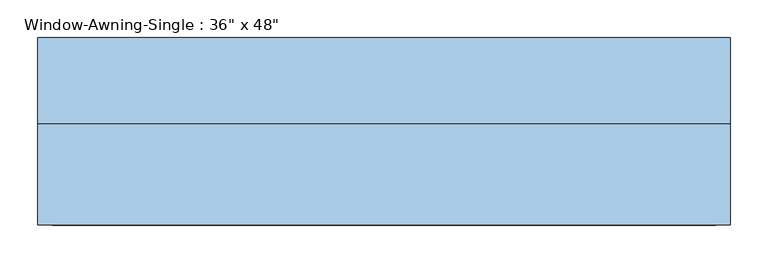
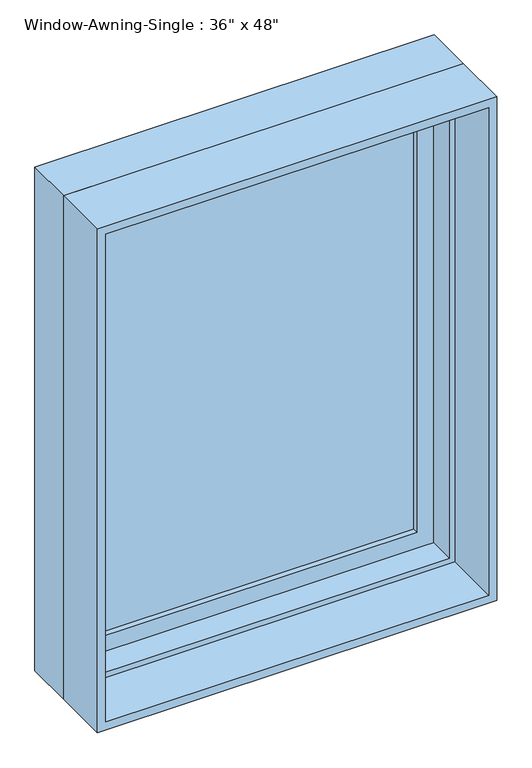
"""IFC4 building model written with IfcOpenShell, lengths in millimetres: window geometry."""

from ifc_helpers import new_model, si_unit, frame, origin, place, context, project, spatial, polyline, outline, extrude, faceted_brep, source, transform, mapped, element, save


def window_272f20d6(model_context):
    return source(origin(), model_context, "Body", "SolidModel", [
        extrude(outline(polyline([(2133.6, -457.2), (914.4, -457.2), (914.4, 457.2), (2133.6, 457.2), (2133.6, -457.2)]), holes=[polyline([(2114.55, -438.15), (2114.55, 438.15), (933.45, 438.15), (933.45, -438.15), (2114.55, -438.15)])]), frame((0.0, -114.3, 0.0), z_axis=(0.0, 1.0, 0.0), x_axis=(0.0, 0.0, 1.0)), (0.0, 0.0, 1.0), 133.35),
        extrude(outline(polyline([(927.1, -444.5), (927.1, 444.5), (2120.9, 444.5), (2120.9, -444.5), (927.1, -444.5)]), holes=[polyline([(2063.75, -387.35), (2063.75, 387.35), (984.25, 387.35), (984.25, -387.35), (2063.75, -387.35)])]), frame((0.0, 82.55, 0.0), z_axis=(0.0, 1.0, 0.0), x_axis=(0.0, 0.0, 1.0)), (0.0, 0.0, 1.0), 44.45),
        extrude(outline(polyline([(387.35, 114.3), (387.35, 107.95), (-387.35, 107.95), (-387.35, 114.3), (387.35, 114.3)])), frame((0.0, 0.0, 984.25), z_axis=(0.0, 0.0, 1.0), x_axis=(1.0, 0.0, 0.0)), (0.0, 0.0, 1.0), 1079.5),
        extrude(outline(polyline([(387.35, 101.6), (387.35, 95.25), (-387.35, 95.25), (-387.35, 101.6), (387.35, 101.6)])), frame((0.0, 0.0, 984.25), z_axis=(0.0, 0.0, 1.0), x_axis=(1.0, 0.0, 0.0)), (0.0, 0.0, 1.0), 1079.5),
        faceted_brep([(444.5, 82.55, 927.1), (444.5, 133.35, 927.1), (-444.5, 133.35, 927.1), (-444.5, 82.55, 927.1), (425.45, 19.05, 946.15), (425.45, 82.55, 946.15), (-425.45, 82.55, 946.15), (-425.45, 19.05, 946.15), (457.2, 133.35, 914.4), (457.2, 19.05, 914.4), (-457.2, 19.05, 914.4), (-457.2, 133.35, 914.4), (-444.5, 133.35, 2120.9), (-444.5, 82.55, 2120.9), (-425.45, 82.55, 2101.85), (-425.45, 19.05, 2101.85), (-457.2, 19.05, 2133.6), (-457.2, 133.35, 2133.6), (444.5, 133.35, 2120.9), (444.5, 82.55, 2120.9), (425.45, 82.55, 2101.85), (425.45, 19.05, 2101.85), (457.2, 19.05, 2133.6), (457.2, 133.35, 2133.6)], [[[0, 1, 2, 3]], [[4, 5, 6, 7]], [[8, 9, 10, 11]], [[3, 2, 12, 13]], [[7, 6, 14, 15]], [[11, 10, 16, 17]], [[13, 12, 18, 19]], [[15, 14, 20, 21]], [[17, 16, 22, 23]], [[11, 17, 23, 8], [1, 18, 12, 2]], [[19, 18, 1, 0]], [[3, 13, 19, 0], [5, 20, 14, 6]], [[21, 20, 5, 4]], [[9, 22, 16, 10], [7, 15, 21, 4]], [[23, 22, 9, 8]]]),
    ])


if __name__ == "__main__":
    model = new_model("IFC4")
    model_context = context("Model", 3, world=origin())
    ifc_project = project(units=[si_unit("LENGTHUNIT", "METRE", prefix="MILLI")], contexts=[model_context])
    site = spatial("IfcSite", under=ifc_project)
    building = spatial("IfcBuilding", under=site)
    placement = place(None, origin())
    window_shape = window_272f20d6(model_context)
    element("IfcWindow", 1, ObjectType="Window-Awning-Single : 36\" x 48\"", at=placement, inside=building, context=model_context, shape_type="MappedRepresentation", body=[
        mapped(window_shape, transform((0.0, 0.0, 0.0), x_axis=(1.0, 0.0, 0.0), y_axis=(0.0, 1.0, 0.0), z_axis=(0.0, 0.0, 1.0))),
    ])
    save(model, "model.ifc")

# Revit data of these elements
# Type "Window-Awning-Single : 36\" x 48\""
#   Type Mark = "20"
#   Fire Rating = "0.5h"
#   Assembly Code = "B2020100"
#   Analytic Construction = "Double glazing - domestic"
#   Window Inset [instance default] = 0' - 0"
#   Wall Thickness [instance default] = 0' - 6"
#   Visual Light Transmittance = 0.81
#   Thermal Resistance (R) = 1.8146 (h·ft²·°F)/BTU
#   Solar Heat Gain Coefficient = 0.76
#   Rough Width = 3' - 0 1/2"
#   Rough Height = 4' - 0 1/2"
#   Interior Wall Closure [instance default] = 0' - 2 1/4"
#   Height = 4' - 0"
#   Heat Transfer Coefficient (U) = 0.5511 BTU/(h·ft²·°F)
#   Frame Extension [instance default] = 0' - 0 1/4"
#   Exterior Wall Closure [instance default] = 0' - 1 1/4"
#   Extension Jamb [instance default] = 0' - 2 1/4"
#   Default Sill Height = 3' - 0"
#   Width = 3' - 0"
#   Muntin Visibility = yes
#   Interior Trim Visibility [instance default] = yes
#   Exterior Trim Visibility [instance default] = yes
#   Extension Jamb Visibility [instance default] = yes
#   Muntin Pattern = Muntin Pattern_2x2 : Muntin Pattern_2x2
#   Interior Trim Material = Wood - Stained
#   Interior Trim = Trim-Window-Interior-Flat : Picture Frame
#   Interior Frame Material = Wood - Stained
#   Glass Panel Material = Glass
#   Exterior Trim Material = Clad - White
#   Exterior Trim = Trim-Window-Exterior-Flat : with Sill
#   Exterior Frame Material = Clad - White
#   Wall Closure = (empty or 0)
# Element 1 (IfcWindow, "Window-Awning-Single : 36\" x 48\"")
#   Wall Thickness = 0' - 9"
#   Extension Jamb = 0' - 5 1/4"
#   Materials on its faces: "Wood - Stained", "Glass", "Clad - White"
# Materials
#   "Wood - Stained": class "Wood", colour RGB 224 178 126, transparency 0, Cost = 0
#   "Glass": class "Glass", colour RGB 0 128 192, transparency 0.75, Description = "Soda Lime Glass", Cost = 0
#   "Clad - White": class "Wood", colour RGB 242 242 238, transparency 0, Cost = 0
